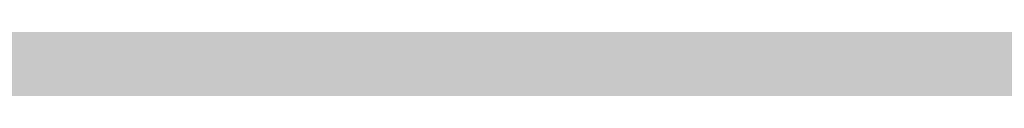
# Model space of a CAD drawing. Units: millimetres. Extents: x -22994 to 29398, y -19990 to 20176.
# Tile 95 of 135: x 229.428 to 230.597, y 84.498 to 84.556. Entities that reach past the tile are written whole.
import ezdxf
from ezdxf import colors
from ezdxf.entities.mleader import LeaderData, LeaderLine
from ezdxf.math import Vec2, Vec3

# ---------------------------------------------------------------- set-up
doc = ezdxf.new("R2010")
doc.units = ezdxf.units.MM
doc.header["$MEASUREMENT"] = 0
for name, color, linetype, lineweight in [('M-ANNO-TEXT', 7, 'Continuous', 25), ('M-DIMS', 2, 'Continuous', 18), ('M-EQPM-PATT', 7, 'Continuous', 18)]:
    doc.layers.add(name, color=color, linetype=linetype, lineweight=lineweight)
doc.styles.get("Standard").update_dxf_attribs({"font": 'arial.ttf'})
doc.dimstyles.get("Standard").update_dxf_attribs({"dimtxt": 0.18, "dimasz": 10000, "dimexe": 0.18, "dimexo": 0.0625, "dimgap": 0.09, "dimtad": 0, "dimtih": 1, "dimtoh": 1, "dimdec": 0, "dimzin": 0, "dimdsep": 46, "dimtxsty": 'Standard', "dimcen": 0.09, "dimadec": 0, "dimazin": 0, "dimtfac": 1, "dimtdec": 0, "dimtofl": 0, "dimtmove": 0, "dimatfit": 3, "dimfxl": 1, "dimtolj": 1, "dimtzin": 0, "dimlwd": 30, "dimarcsym": 0})

# ---------------------------------------------------------------- blocks, each defined once
blk = doc.blocks.new('*D2')
at = {"layer": 'Defpoints', "color": 0, "transparency": 16777216}
for p in [(6.6773, 10.2713), (290.852, 10.2713), (290.852, -5.0787)]:
    blk.add_point(p, dxfattribs=at)
at = {"layer": 'M-DIMS', "color": 0, "lineweight": -2, "transparency": 16777216}
for p, q in [((6.6773, 10.2088), (6.6773, -5.2587)), ((290.852, 10.2088), (290.852, -5.2587))]:
    blk.add_line(p, q, dxfattribs=at)
at = {"layer": 'M-DIMS', "color": 0, "lineweight": 30, "transparency": 16777216}
for p, q in [((-9993.3227, -5.0787), (-19993.3227, -5.0787)), ((10290.852, -5.0787), (20290.852, -5.0787))]:
    blk.add_line(p, q, dxfattribs=at)
at = {"layer": 'M-DIMS', "color": 0, "transparency": 16777216}
for points in [[(-9993.3227, 1661.5879), (-9993.3227, -1671.7454), (6.6773, -5.0787)], [(10290.852, 1661.5879), (10290.852, -1671.7454), (290.852, -5.0787)]]:
    blk.add_solid(points, dxfattribs=at)
at = {"layer": 'M-DIMS', "color": 0, "transparency": 16777216, "insert": (148.7647, -5.0787), "char_height": 0.18, "attachment_point": 5}
blk.add_mtext('\\A1;284.2', dxfattribs=at)
blk = doc.blocks.new('*D3')
at = {"layer": 'Defpoints', "color": 0, "transparency": 16777216}
for p in [(110.2647, 204.1654), (110.2647, 176.3662), (95.8327, 127.967)]:
    blk.add_point(p, dxfattribs=at)
at = {"layer": 'M-DIMS', "color": 0, "lineweight": -2, "transparency": 16777216}
for p, q in [((95.8327, 128.0295), (95.8327, 204.3454)), ((110.2647, 176.4287), (110.2647, 204.3454))]:
    blk.add_line(p, q, dxfattribs=at)
at = {"layer": 'M-DIMS', "color": 0, "lineweight": 30, "transparency": 16777216}
for p, q in [((-9904.1673, 204.1654), (-19904.1673, 204.1654)), ((10110.2647, 204.1654), (20110.2647, 204.1654))]:
    blk.add_line(p, q, dxfattribs=at)
at = {"layer": 'M-DIMS', "color": 0, "transparency": 16777216}
for points in [[(-9904.1673, 1870.8321), (-9904.1673, -1462.5013), (95.8327, 204.1654)], [(10110.2647, 1870.8321), (10110.2647, -1462.5013), (110.2647, 204.1654)]]:
    blk.add_solid(points, dxfattribs=at)
at = {"layer": 'M-DIMS', "color": 0, "transparency": 16777216, "insert": (103.0487, 204.1654), "char_height": 0.18, "attachment_point": 5}
blk.add_mtext('\\A1;14.432', dxfattribs=at)
blk = doc.blocks.new('*D4')
at = {"layer": 'Defpoints', "color": 0, "transparency": 16777216}
for p in [(116.2647, 204.1654), (110.2647, 176.3662), (116.2647, 176.3662)]:
    blk.add_point(p, dxfattribs=at)
at = {"layer": 'M-DIMS', "color": 0, "lineweight": -2, "transparency": 16777216}
for p, q in [((110.2647, 176.4287), (110.2647, 204.3454)), ((116.2647, 176.4287), (116.2647, 204.3454))]:
    blk.add_line(p, q, dxfattribs=at)
at = {"layer": 'M-DIMS', "color": 0, "lineweight": 30, "transparency": 16777216}
for p, q in [((-9889.7353, 204.1654), (-19889.7353, 204.1654)), ((10116.2647, 204.1654), (20116.2647, 204.1654))]:
    blk.add_line(p, q, dxfattribs=at)
at = {"layer": 'M-DIMS', "color": 0, "transparency": 16777216}
for points in [[(-9889.7353, 1870.8321), (-9889.7353, -1462.5013), (110.2647, 204.1654)], [(10116.2647, 1870.8321), (10116.2647, -1462.5013), (116.2647, 204.1654)]]:
    blk.add_solid(points, dxfattribs=at)
at = {"layer": 'M-DIMS', "color": 0, "transparency": 16777216, "insert": (113.2647, 204.1654), "char_height": 0.18, "attachment_point": 5}
blk.add_mtext('\\A1;6', dxfattribs=at)
blk = doc.blocks.new('*D5')
at = {"layer": 'Defpoints', "color": 0, "transparency": 16777216}
for p in [(181.2647, 204.1654), (116.2647, 176.3662), (181.2647, 176.3662)]:
    blk.add_point(p, dxfattribs=at)
at = {"layer": 'M-DIMS', "color": 0, "lineweight": -2, "transparency": 16777216}
for p, q in [((116.2647, 176.4287), (116.2647, 204.3454)), ((181.2647, 176.4287), (181.2647, 204.3454))]:
    blk.add_line(p, q, dxfattribs=at)
at = {"layer": 'M-DIMS', "color": 0, "lineweight": 30, "transparency": 16777216}
for p, q in [((-9883.7353, 204.1654), (-19883.7353, 204.1654)), ((10181.2647, 204.1654), (20181.2647, 204.1654))]:
    blk.add_line(p, q, dxfattribs=at)
at = {"layer": 'M-DIMS', "color": 0, "transparency": 16777216}
for points in [[(-9883.7353, 1870.8321), (-9883.7353, -1462.5013), (116.2647, 204.1654)], [(10181.2647, 1870.8321), (10181.2647, -1462.5013), (181.2647, 204.1654)]]:
    blk.add_solid(points, dxfattribs=at)
at = {"layer": 'M-DIMS', "color": 0, "transparency": 16777216, "insert": (148.7647, 204.1654), "char_height": 0.18, "attachment_point": 5}
blk.add_mtext('\\A1;65', dxfattribs=at)
blk = doc.blocks.new('*D6')
at = {"layer": 'Defpoints', "color": 0, "transparency": 16777216}
for p in [(187.2647, 204.1654), (181.2647, 176.3662), (187.2647, 176.3662)]:
    blk.add_point(p, dxfattribs=at)
at = {"layer": 'M-DIMS', "color": 0, "lineweight": -2, "transparency": 16777216}
for p, q in [((181.2647, 176.4287), (181.2647, 204.3454)), ((187.2647, 176.4287), (187.2647, 204.3454))]:
    blk.add_line(p, q, dxfattribs=at)
at = {"layer": 'M-DIMS', "color": 0, "lineweight": 30, "transparency": 16777216}
for p, q in [((-9818.7353, 204.1654), (-19818.7353, 204.1654)), ((10187.2647, 204.1654), (20187.2647, 204.1654))]:
    blk.add_line(p, q, dxfattribs=at)
at = {"layer": 'M-DIMS', "color": 0, "transparency": 16777216}
for points in [[(-9818.7353, 1870.8321), (-9818.7353, -1462.5013), (181.2647, 204.1654)], [(10187.2647, 1870.8321), (10187.2647, -1462.5013), (187.2647, 204.1654)]]:
    blk.add_solid(points, dxfattribs=at)
at = {"layer": 'M-DIMS', "color": 0, "transparency": 16777216, "insert": (184.2647, 204.1654), "char_height": 0.18, "attachment_point": 5}
blk.add_mtext('\\A1;6', dxfattribs=at)
blk = doc.blocks.new('*D7')
at = {"layer": 'Defpoints', "color": 0, "transparency": 16777216}
for p in [(201.6967, 204.1654), (187.2647, 176.3662), (201.6967, 127.967)]:
    blk.add_point(p, dxfattribs=at)
at = {"layer": 'M-DIMS', "color": 0, "lineweight": -2, "transparency": 16777216}
for p, q in [((187.2647, 176.4287), (187.2647, 204.3454)), ((201.6967, 128.0295), (201.6967, 204.3454))]:
    blk.add_line(p, q, dxfattribs=at)
at = {"layer": 'M-DIMS', "color": 0, "lineweight": 30, "transparency": 16777216}
for p, q in [((-9812.7353, 204.1654), (-19812.7353, 204.1654)), ((10201.6967, 204.1654), (20201.6967, 204.1654))]:
    blk.add_line(p, q, dxfattribs=at)
at = {"layer": 'M-DIMS', "color": 0, "transparency": 16777216}
for points in [[(-9812.7353, 1870.8321), (-9812.7353, -1462.5013), (187.2647, 204.1654)], [(10201.6967, 1870.8321), (10201.6967, -1462.5013), (201.6967, 204.1654)]]:
    blk.add_solid(points, dxfattribs=at)
at = {"layer": 'M-DIMS', "color": 0, "transparency": 16777216, "insert": (194.4807, 204.1654), "char_height": 0.18, "attachment_point": 5}
blk.add_mtext('\\A1;14.432', dxfattribs=at)
blk = doc.blocks.new('*D8')
at = {"layer": 'Defpoints', "color": 0, "transparency": 16777216}
for p in [(227.6485, 204.1654), (227.6485, 146.7296), (201.6967, 127.967)]:
    blk.add_point(p, dxfattribs=at)
at = {"layer": 'M-DIMS', "color": 0, "lineweight": -2, "transparency": 16777216}
for p, q in [((201.6967, 128.0295), (201.6967, 204.3454)), ((227.6485, 146.7921), (227.6485, 204.3454))]:
    blk.add_line(p, q, dxfattribs=at)
at = {"layer": 'M-DIMS', "color": 0, "lineweight": 30, "transparency": 16777216}
for p, q in [((-9798.3033, 204.1654), (-19798.3033, 204.1654)), ((10227.6485, 204.1654), (20227.6485, 204.1654))]:
    blk.add_line(p, q, dxfattribs=at)
at = {"layer": 'M-DIMS', "color": 0, "transparency": 16777216}
for points in [[(-9798.3033, 1870.8321), (-9798.3033, -1462.5013), (201.6967, 204.1654)], [(10227.6485, 1870.8321), (10227.6485, -1462.5013), (227.6485, 204.1654)]]:
    blk.add_solid(points, dxfattribs=at)
at = {"layer": 'M-DIMS', "color": 0, "transparency": 16777216, "insert": (214.6726, 204.1654), "char_height": 0.18, "attachment_point": 5}
blk.add_mtext('\\A1;25.95', dxfattribs=at)
blk = doc.blocks.new('*D9')
at = {"layer": 'Defpoints', "color": 0, "transparency": 16777216}
for p in [(187.2647, 176.3662), (306.202, 176.3662), (290.852, 10.2713)]:
    blk.add_point(p, dxfattribs=at)
at = {"layer": 'M-DIMS', "color": 0, "lineweight": 30, "transparency": 16777216}
for p, q in [((306.202, 10176.3662), (306.202, 20176.3662)), ((306.202, -9989.7287), (306.202, -19989.7287))]:
    blk.add_line(p, q, dxfattribs=at)
at = {"layer": 'M-DIMS', "color": 0, "lineweight": -2, "transparency": 16777216}
for p, q in [((187.3272, 176.3662), (306.382, 176.3662)), ((290.9145, 10.2713), (306.382, 10.2713))]:
    blk.add_line(p, q, dxfattribs=at)
at = {"layer": 'M-DIMS', "color": 0, "transparency": 16777216}
for points in [[(-1360.4646, 10176.3662), (1972.8687, 10176.3662), (306.202, 176.3662)], [(-1360.4646, -9989.7287), (1972.8687, -9989.7287), (306.202, 10.2713)]]:
    blk.add_solid(points, dxfattribs=at)
at = {"layer": 'M-DIMS', "color": 0, "transparency": 16777216, "insert": (306.202, 93.3187), "char_height": 0.18, "attachment_point": 5}
blk.add_mtext('\\A1;166.1', dxfattribs=at)
blk = doc.blocks.new('*D10')
at = {"layer": 'Defpoints', "color": 0, "transparency": 16777216}
for p in [(125.6498, 136.0713), (133.3459, 136.0713), (133.3459, -5.0787)]:
    blk.add_point(p, dxfattribs=at)
at = {"layer": 'M-DIMS', "color": 0, "lineweight": -2, "transparency": 16777216}
for p, q in [((125.6498, 136.0088), (125.6498, -5.2587)), ((133.3459, 136.0088), (133.3459, -5.2587))]:
    blk.add_line(p, q, dxfattribs=at)
at = {"layer": 'M-DIMS', "color": 0, "lineweight": 30, "transparency": 16777216}
for p, q in [((-9874.3502, -5.0787), (-19874.3502, -5.0787)), ((10133.3459, -5.0787), (20133.3459, -5.0787))]:
    blk.add_line(p, q, dxfattribs=at)
at = {"layer": 'M-DIMS', "color": 0, "transparency": 16777216}
for points in [[(-9874.3502, 1661.5879), (-9874.3502, -1671.7454), (125.6498, -5.0787)], [(10133.3459, 1661.5879), (10133.3459, -1671.7454), (133.3459, -5.0787)]]:
    blk.add_solid(points, dxfattribs=at)
at = {"layer": 'M-DIMS', "color": 0, "transparency": 16777216, "insert": (129.4978, -5.0787), "char_height": 0.18, "attachment_point": 5}
blk.add_mtext('\\A1;7.696', dxfattribs=at)
blk = doc.blocks.new('*D11')
at = {"layer": 'Defpoints', "color": 0, "transparency": 16777216}
for p in [(133.3459, 136.0713), (135.6498, 136.0713), (135.6498, -5.0787)]:
    blk.add_point(p, dxfattribs=at)
at = {"layer": 'M-DIMS', "color": 0, "lineweight": -2, "transparency": 16777216}
for p, q in [((133.3459, 136.0088), (133.3459, -5.2587)), ((135.6498, 136.0088), (135.6498, -5.2587))]:
    blk.add_line(p, q, dxfattribs=at)
at = {"layer": 'M-DIMS', "color": 0, "lineweight": 30, "transparency": 16777216}
for p, q in [((-9866.6541, -5.0787), (-19866.6541, -5.0787)), ((10135.6498, -5.0787), (20135.6498, -5.0787))]:
    blk.add_line(p, q, dxfattribs=at)
at = {"layer": 'M-DIMS', "color": 0, "transparency": 16777216}
for points in [[(-9866.6541, 1661.5879), (-9866.6541, -1671.7454), (133.3459, -5.0787)], [(10135.6498, 1661.5879), (10135.6498, -1671.7454), (135.6498, -5.0787)]]:
    blk.add_solid(points, dxfattribs=at)
at = {"layer": 'M-DIMS', "color": 0, "transparency": 16777216, "insert": (134.4978, -5.0787), "char_height": 0.18, "attachment_point": 5}
blk.add_mtext('\\A1;2.304', dxfattribs=at)
blk = doc.blocks.new('*D12')
at = {"layer": 'Defpoints', "color": 0, "transparency": 16777216}
for p in [(135.6498, 136.0713), (145.6498, 136.0713), (145.6498, -5.0787)]:
    blk.add_point(p, dxfattribs=at)
at = {"layer": 'M-DIMS', "color": 0, "lineweight": -2, "transparency": 16777216}
for p, q in [((135.6498, 136.0088), (135.6498, -5.2587)), ((145.6498, 136.0088), (145.6498, -5.2587))]:
    blk.add_line(p, q, dxfattribs=at)
at = {"layer": 'M-DIMS', "color": 0, "lineweight": 30, "transparency": 16777216}
for p, q in [((-9864.3502, -5.0787), (-19864.3502, -5.0787)), ((10145.6498, -5.0787), (20145.6498, -5.0787))]:
    blk.add_line(p, q, dxfattribs=at)
at = {"layer": 'M-DIMS', "color": 0, "transparency": 16777216}
for points in [[(-9864.3502, 1661.5879), (-9864.3502, -1671.7454), (135.6498, -5.0787)], [(10145.6498, 1661.5879), (10145.6498, -1671.7454), (145.6498, -5.0787)]]:
    blk.add_solid(points, dxfattribs=at)
at = {"layer": 'M-DIMS', "color": 0, "transparency": 16777216, "insert": (140.6498, -5.0787), "char_height": 0.18, "attachment_point": 5}
blk.add_mtext('\\A1;10', dxfattribs=at)
blk = doc.blocks.new('*D13')
at = {"layer": 'Defpoints', "color": 0, "transparency": 16777216}
for p in [(145.6498, 136.0713), (155.6498, 136.0713), (155.6498, -5.0787)]:
    blk.add_point(p, dxfattribs=at)
at = {"layer": 'M-DIMS', "color": 0, "lineweight": -2, "transparency": 16777216}
for p, q in [((145.6498, 136.0088), (145.6498, -5.2587)), ((155.6498, 136.0088), (155.6498, -5.2587))]:
    blk.add_line(p, q, dxfattribs=at)
at = {"layer": 'M-DIMS', "color": 0, "lineweight": 30, "transparency": 16777216}
for p, q in [((-9854.3502, -5.0787), (-19854.3502, -5.0787)), ((10155.6498, -5.0787), (20155.6498, -5.0787))]:
    blk.add_line(p, q, dxfattribs=at)
at = {"layer": 'M-DIMS', "color": 0, "transparency": 16777216}
for points in [[(-9854.3502, 1661.5879), (-9854.3502, -1671.7454), (145.6498, -5.0787)], [(10155.6498, 1661.5879), (10155.6498, -1671.7454), (155.6498, -5.0787)]]:
    blk.add_solid(points, dxfattribs=at)
at = {"layer": 'M-DIMS', "color": 0, "transparency": 16777216, "insert": (150.6498, -5.0787), "char_height": 0.18, "attachment_point": 5}
blk.add_mtext('\\A1;10', dxfattribs=at)
blk = doc.blocks.new('*D14')
at = {"layer": 'Defpoints', "color": 0, "transparency": 16777216}
for p in [(155.6498, 136.0713), (165.6498, 136.0713), (165.6498, -5.0787)]:
    blk.add_point(p, dxfattribs=at)
at = {"layer": 'M-DIMS', "color": 0, "lineweight": -2, "transparency": 16777216}
for p, q in [((155.6498, 136.0088), (155.6498, -5.2587)), ((165.6498, 136.0088), (165.6498, -5.2587))]:
    blk.add_line(p, q, dxfattribs=at)
at = {"layer": 'M-DIMS', "color": 0, "lineweight": 30, "transparency": 16777216}
for p, q in [((-9844.3502, -5.0787), (-19844.3502, -5.0787)), ((10165.6498, -5.0787), (20165.6498, -5.0787))]:
    blk.add_line(p, q, dxfattribs=at)
at = {"layer": 'M-DIMS', "color": 0, "transparency": 16777216}
for points in [[(-9844.3502, 1661.5879), (-9844.3502, -1671.7454), (155.6498, -5.0787)], [(10165.6498, 1661.5879), (10165.6498, -1671.7454), (165.6498, -5.0787)]]:
    blk.add_solid(points, dxfattribs=at)
at = {"layer": 'M-DIMS', "color": 0, "transparency": 16777216, "insert": (160.6498, -5.0787), "char_height": 0.18, "attachment_point": 5}
blk.add_mtext('\\A1;10', dxfattribs=at)
blk = doc.blocks.new('*D15')
at = {"layer": 'Defpoints', "color": 0, "transparency": 16777216}
for p in [(173.3459, 154.788), (173.3459, 136.0713), (306.202, 136.0713)]:
    blk.add_point(p, dxfattribs=at)
at = {"layer": 'M-DIMS', "color": 0, "lineweight": 30, "transparency": 16777216}
for p, q in [((306.202, 10154.788), (306.202, 20154.788)), ((306.202, -9863.9287), (306.202, -19863.9287))]:
    blk.add_line(p, q, dxfattribs=at)
at = {"layer": 'M-DIMS', "color": 0, "lineweight": -2, "transparency": 16777216}
for p, q in [((173.4084, 154.788), (306.382, 154.788)), ((173.4084, 136.0713), (306.382, 136.0713))]:
    blk.add_line(p, q, dxfattribs=at)
at = {"layer": 'M-DIMS', "color": 0, "transparency": 16777216}
for points in [[(-1360.4646, 10154.788), (1972.8687, 10154.788), (306.202, 154.788)], [(-1360.4646, -9863.9287), (1972.8687, -9863.9287), (306.202, 136.0713)]]:
    blk.add_solid(points, dxfattribs=at)
at = {"layer": 'M-DIMS', "color": 0, "transparency": 16777216, "insert": (306.202, 145.4297), "char_height": 0.18, "attachment_point": 5}
blk.add_mtext('\\A1;18.717', dxfattribs=at)
blk = doc.blocks.new('*D16')
at = {"layer": 'Defpoints', "color": 0, "transparency": 16777216}
for p in [(120.1702, 204.1654), (110.4658, 48.0349), (120.1702, 48.0349)]:
    blk.add_point(p, dxfattribs=at)
at = {"layer": 'M-DIMS', "color": 0, "lineweight": -2, "transparency": 16777216}
for p, q in [((110.4658, 48.0974), (110.4658, 204.3454)), ((120.1702, 48.0974), (120.1702, 204.3454))]:
    blk.add_line(p, q, dxfattribs=at)
at = {"layer": 'M-DIMS', "color": 0, "lineweight": 30, "transparency": 16777216}
for p, q in [((-9889.5342, 204.1654), (-19889.5342, 204.1654)), ((10120.1702, 204.1654), (20120.1702, 204.1654))]:
    blk.add_line(p, q, dxfattribs=at)
at = {"layer": 'M-DIMS', "color": 0, "transparency": 16777216}
for points in [[(-9889.5342, 1870.8321), (-9889.5342, -1462.5013), (110.4658, 204.1654)], [(10120.1702, 1870.8321), (10120.1702, -1462.5013), (120.1702, 204.1654)]]:
    blk.add_solid(points, dxfattribs=at)
at = {"layer": 'M-DIMS', "color": 0, "transparency": 16777216, "insert": (115.318, 204.1654), "char_height": 0.18, "attachment_point": 5}
blk.add_mtext('\\A1;9.704', dxfattribs=at)
blk = doc.blocks.new('*D17')
at = {"layer": 'Defpoints', "color": 0, "transparency": 16777216}
for p in [(126.1702, 204.1654), (120.1702, 48.0349), (126.1702, 48.0349)]:
    blk.add_point(p, dxfattribs=at)
at = {"layer": 'M-DIMS', "color": 0, "lineweight": -2, "transparency": 16777216}
for p, q in [((120.1702, 48.0974), (120.1702, 204.3454)), ((126.1702, 48.0974), (126.1702, 204.3454))]:
    blk.add_line(p, q, dxfattribs=at)
at = {"layer": 'M-DIMS', "color": 0, "lineweight": 30, "transparency": 16777216}
for p, q in [((-9879.8298, 204.1654), (-19879.8298, 204.1654)), ((10126.1702, 204.1654), (20126.1702, 204.1654))]:
    blk.add_line(p, q, dxfattribs=at)
at = {"layer": 'M-DIMS', "color": 0, "transparency": 16777216}
for points in [[(-9879.8298, 1870.8321), (-9879.8298, -1462.5013), (120.1702, 204.1654)], [(10126.1702, 1870.8321), (10126.1702, -1462.5013), (126.1702, 204.1654)]]:
    blk.add_solid(points, dxfattribs=at)
at = {"layer": 'M-DIMS', "color": 0, "transparency": 16777216, "insert": (123.1702, 204.1654), "char_height": 0.18, "attachment_point": 5}
blk.add_mtext('\\A1;6', dxfattribs=at)
blk = doc.blocks.new('*D18')
at = {"layer": 'Defpoints', "color": 0, "transparency": 16777216}
for p in [(132.1702, 204.1654), (126.1702, 48.0349), (132.1702, 48.0349)]:
    blk.add_point(p, dxfattribs=at)
at = {"layer": 'M-DIMS', "color": 0, "lineweight": -2, "transparency": 16777216}
for p, q in [((126.1702, 48.0974), (126.1702, 204.3454)), ((132.1702, 48.0974), (132.1702, 204.3454))]:
    blk.add_line(p, q, dxfattribs=at)
at = {"layer": 'M-DIMS', "color": 0, "lineweight": 30, "transparency": 16777216}
for p, q in [((-9873.8298, 204.1654), (-19873.8298, 204.1654)), ((10132.1702, 204.1654), (20132.1702, 204.1654))]:
    blk.add_line(p, q, dxfattribs=at)
at = {"layer": 'M-DIMS', "color": 0, "transparency": 16777216}
for points in [[(-9873.8298, 1870.8321), (-9873.8298, -1462.5013), (126.1702, 204.1654)], [(10132.1702, 1870.8321), (10132.1702, -1462.5013), (132.1702, 204.1654)]]:
    blk.add_solid(points, dxfattribs=at)
at = {"layer": 'M-DIMS', "color": 0, "transparency": 16777216, "insert": (129.1702, 204.1654), "char_height": 0.18, "attachment_point": 5}
blk.add_mtext('\\A1;6', dxfattribs=at)
blk = doc.blocks.new('*D19')
at = {"layer": 'Defpoints', "color": 0, "transparency": 16777216}
for p in [(138.1702, 204.1654), (132.1702, 48.0349), (138.1702, 48.0349)]:
    blk.add_point(p, dxfattribs=at)
at = {"layer": 'M-DIMS', "color": 0, "lineweight": -2, "transparency": 16777216}
for p, q in [((132.1702, 48.0974), (132.1702, 204.3454)), ((138.1702, 48.0974), (138.1702, 204.3454))]:
    blk.add_line(p, q, dxfattribs=at)
at = {"layer": 'M-DIMS', "color": 0, "lineweight": 30, "transparency": 16777216}
for p, q in [((-9867.8298, 204.1654), (-19867.8298, 204.1654)), ((10138.1702, 204.1654), (20138.1702, 204.1654))]:
    blk.add_line(p, q, dxfattribs=at)
at = {"layer": 'M-DIMS', "color": 0, "transparency": 16777216}
for points in [[(-9867.8298, 1870.8321), (-9867.8298, -1462.5013), (132.1702, 204.1654)], [(10138.1702, 1870.8321), (10138.1702, -1462.5013), (138.1702, 204.1654)]]:
    blk.add_solid(points, dxfattribs=at)
at = {"layer": 'M-DIMS', "color": 0, "transparency": 16777216, "insert": (135.1702, 204.1654), "char_height": 0.18, "attachment_point": 5}
blk.add_mtext('\\A1;6', dxfattribs=at)
blk = doc.blocks.new('*D20')
at = {"layer": 'Defpoints', "color": 0, "transparency": 16777216}
for p in [(144.1702, 204.1654), (138.1702, 48.0349), (144.1702, 48.0349)]:
    blk.add_point(p, dxfattribs=at)
at = {"layer": 'M-DIMS', "color": 0, "lineweight": -2, "transparency": 16777216}
for p, q in [((138.1702, 48.0974), (138.1702, 204.3454)), ((144.1702, 48.0974), (144.1702, 204.3454))]:
    blk.add_line(p, q, dxfattribs=at)
at = {"layer": 'M-DIMS', "color": 0, "lineweight": 30, "transparency": 16777216}
for p, q in [((-9861.8298, 204.1654), (-19861.8298, 204.1654)), ((10144.1702, 204.1654), (20144.1702, 204.1654))]:
    blk.add_line(p, q, dxfattribs=at)
at = {"layer": 'M-DIMS', "color": 0, "transparency": 16777216}
for points in [[(-9861.8298, 1870.8321), (-9861.8298, -1462.5013), (138.1702, 204.1654)], [(10144.1702, 1870.8321), (10144.1702, -1462.5013), (144.1702, 204.1654)]]:
    blk.add_solid(points, dxfattribs=at)
at = {"layer": 'M-DIMS', "color": 0, "transparency": 16777216, "insert": (141.1702, 204.1654), "char_height": 0.18, "attachment_point": 5}
blk.add_mtext('\\A1;6', dxfattribs=at)
blk = doc.blocks.new('*D21')
at = {"layer": 'Defpoints', "color": 0, "transparency": 16777216}
for p in [(149.1157, 204.1654), (144.1702, 48.0349), (149.1157, 48.0349)]:
    blk.add_point(p, dxfattribs=at)
at = {"layer": 'M-DIMS', "color": 0, "lineweight": -2, "transparency": 16777216}
for p, q in [((144.1702, 48.0974), (144.1702, 204.3454)), ((149.1157, 48.0974), (149.1157, 204.3454))]:
    blk.add_line(p, q, dxfattribs=at)
at = {"layer": 'M-DIMS', "color": 0, "lineweight": 30, "transparency": 16777216}
for p, q in [((-9855.8298, 204.1654), (-19855.8298, 204.1654)), ((10149.1157, 204.1654), (20149.1157, 204.1654))]:
    blk.add_line(p, q, dxfattribs=at)
at = {"layer": 'M-DIMS', "color": 0, "transparency": 16777216}
for points in [[(-9855.8298, 1870.8321), (-9855.8298, -1462.5013), (144.1702, 204.1654)], [(10149.1157, 1870.8321), (10149.1157, -1462.5013), (149.1157, 204.1654)]]:
    blk.add_solid(points, dxfattribs=at)
at = {"layer": 'M-DIMS', "color": 0, "transparency": 16777216, "insert": (146.6429, 204.1654), "char_height": 0.18, "attachment_point": 5}
blk.add_mtext('\\A1;4.945', dxfattribs=at)
blk = doc.blocks.new('*D22')
at = {"layer": 'Defpoints', "color": 0, "transparency": 16777216}
for p in [(149.1157, 30.9895), (155.1157, 30.9895), (155.1157, -5.0787)]:
    blk.add_point(p, dxfattribs=at)
at = {"layer": 'M-DIMS', "color": 0, "lineweight": -2, "transparency": 16777216}
for p, q in [((149.1157, 30.927), (149.1157, -5.2587)), ((155.1157, 30.927), (155.1157, -5.2587))]:
    blk.add_line(p, q, dxfattribs=at)
at = {"layer": 'M-DIMS', "color": 0, "lineweight": 30, "transparency": 16777216}
for p, q in [((-9850.8843, -5.0787), (-19850.8843, -5.0787)), ((10155.1157, -5.0787), (20155.1157, -5.0787))]:
    blk.add_line(p, q, dxfattribs=at)
at = {"layer": 'M-DIMS', "color": 0, "transparency": 16777216}
for points in [[(-9850.8843, 1661.5879), (-9850.8843, -1671.7454), (149.1157, -5.0787)], [(10155.1157, 1661.5879), (10155.1157, -1671.7454), (155.1157, -5.0787)]]:
    blk.add_solid(points, dxfattribs=at)
at = {"layer": 'M-DIMS', "color": 0, "transparency": 16777216, "insert": (152.1157, -5.0787), "char_height": 0.18, "attachment_point": 5}
blk.add_mtext('\\A1;6', dxfattribs=at)
blk = doc.blocks.new('*D23')
at = {"layer": 'Defpoints', "color": 0, "transparency": 16777216}
for p in [(155.1157, 30.9895), (161.1157, 30.9895), (161.1157, -5.0787)]:
    blk.add_point(p, dxfattribs=at)
at = {"layer": 'M-DIMS', "color": 0, "lineweight": -2, "transparency": 16777216}
for p, q in [((155.1157, 30.927), (155.1157, -5.2587)), ((161.1157, 30.927), (161.1157, -5.2587))]:
    blk.add_line(p, q, dxfattribs=at)
at = {"layer": 'M-DIMS', "color": 0, "lineweight": 30, "transparency": 16777216}
for p, q in [((-9844.8843, -5.0787), (-19844.8843, -5.0787)), ((10161.1157, -5.0787), (20161.1157, -5.0787))]:
    blk.add_line(p, q, dxfattribs=at)
at = {"layer": 'M-DIMS', "color": 0, "transparency": 16777216}
for points in [[(-9844.8843, 1661.5879), (-9844.8843, -1671.7454), (155.1157, -5.0787)], [(10161.1157, 1661.5879), (10161.1157, -1671.7454), (161.1157, -5.0787)]]:
    blk.add_solid(points, dxfattribs=at)
at = {"layer": 'M-DIMS', "color": 0, "transparency": 16777216, "insert": (158.1157, -5.0787), "char_height": 0.18, "attachment_point": 5}
blk.add_mtext('\\A1;6', dxfattribs=at)
blk = doc.blocks.new('*D24')
at = {"layer": 'Defpoints', "color": 0, "transparency": 16777216}
for p in [(161.1157, 30.9895), (166.4387, 30.9895), (166.4387, -5.0787)]:
    blk.add_point(p, dxfattribs=at)
at = {"layer": 'M-DIMS', "color": 0, "lineweight": -2, "transparency": 16777216}
for p, q in [((161.1157, 30.927), (161.1157, -5.2587)), ((166.4387, 30.927), (166.4387, -5.2587))]:
    blk.add_line(p, q, dxfattribs=at)
at = {"layer": 'M-DIMS', "color": 0, "lineweight": 30, "transparency": 16777216}
for p, q in [((-9838.8843, -5.0787), (-19838.8843, -5.0787)), ((10166.4387, -5.0787), (20166.4387, -5.0787))]:
    blk.add_line(p, q, dxfattribs=at)
at = {"layer": 'M-DIMS', "color": 0, "transparency": 16777216}
for points in [[(-9838.8843, 1661.5879), (-9838.8843, -1671.7454), (161.1157, -5.0787)], [(10166.4387, 1661.5879), (10166.4387, -1671.7454), (166.4387, -5.0787)]]:
    blk.add_solid(points, dxfattribs=at)
at = {"layer": 'M-DIMS', "color": 0, "transparency": 16777216, "insert": (163.7772, -5.0787), "char_height": 0.18, "attachment_point": 5}
blk.add_mtext('\\A1;5.323', dxfattribs=at)
blk = doc.blocks.new('*D25')
at = {"layer": 'Defpoints', "color": 0, "transparency": 16777216}
for p in [(166.4387, 30.9895), (172.4387, 30.9895), (172.4387, -5.0787)]:
    blk.add_point(p, dxfattribs=at)
at = {"layer": 'M-DIMS', "color": 0, "lineweight": -2, "transparency": 16777216}
for p, q in [((166.4387, 30.927), (166.4387, -5.2587)), ((172.4387, 30.927), (172.4387, -5.2587))]:
    blk.add_line(p, q, dxfattribs=at)
at = {"layer": 'M-DIMS', "color": 0, "lineweight": 30, "transparency": 16777216}
for p, q in [((-9833.5613, -5.0787), (-19833.5613, -5.0787)), ((10172.4387, -5.0787), (20172.4387, -5.0787))]:
    blk.add_line(p, q, dxfattribs=at)
at = {"layer": 'M-DIMS', "color": 0, "transparency": 16777216}
for points in [[(-9833.5613, 1661.5879), (-9833.5613, -1671.7454), (166.4387, -5.0787)], [(10172.4387, 1661.5879), (10172.4387, -1671.7454), (172.4387, -5.0787)]]:
    blk.add_solid(points, dxfattribs=at)
at = {"layer": 'M-DIMS', "color": 0, "transparency": 16777216, "insert": (169.4387, -5.0787), "char_height": 0.18, "attachment_point": 5}
blk.add_mtext('\\A1;6', dxfattribs=at)
blk = doc.blocks.new('*D26')
at = {"layer": 'Defpoints', "color": 0, "transparency": 16777216}
for p in [(172.4387, 30.9895), (178.4387, 30.9895), (178.4387, -5.0787)]:
    blk.add_point(p, dxfattribs=at)
at = {"layer": 'M-DIMS', "color": 0, "lineweight": -2, "transparency": 16777216}
for p, q in [((172.4387, 30.927), (172.4387, -5.2587)), ((178.4387, 30.927), (178.4387, -5.2587))]:
    blk.add_line(p, q, dxfattribs=at)
at = {"layer": 'M-DIMS', "color": 0, "lineweight": 30, "transparency": 16777216}
for p, q in [((-9827.5613, -5.0787), (-19827.5613, -5.0787)), ((10178.4387, -5.0787), (20178.4387, -5.0787))]:
    blk.add_line(p, q, dxfattribs=at)
at = {"layer": 'M-DIMS', "color": 0, "transparency": 16777216}
for points in [[(-9827.5613, 1661.5879), (-9827.5613, -1671.7454), (172.4387, -5.0787)], [(10178.4387, 1661.5879), (10178.4387, -1671.7454), (178.4387, -5.0787)]]:
    blk.add_solid(points, dxfattribs=at)
at = {"layer": 'M-DIMS', "color": 0, "transparency": 16777216, "insert": (175.4387, -5.0787), "char_height": 0.18, "attachment_point": 5}
blk.add_mtext('\\A1;6', dxfattribs=at)
blk = doc.blocks.new('*D27')
at = {"layer": 'Defpoints', "color": 0, "transparency": 16777216}
for p in [(178.4387, 30.9895), (188.1175, 30.9895), (188.1175, -5.0787)]:
    blk.add_point(p, dxfattribs=at)
at = {"layer": 'M-DIMS', "color": 0, "lineweight": -2, "transparency": 16777216}
for p, q in [((178.4387, 30.927), (178.4387, -5.2587)), ((188.1175, 30.927), (188.1175, -5.2587))]:
    blk.add_line(p, q, dxfattribs=at)
at = {"layer": 'M-DIMS', "color": 0, "lineweight": 30, "transparency": 16777216}
for p, q in [((-9821.5613, -5.0787), (-19821.5613, -5.0787)), ((10188.1175, -5.0787), (20188.1175, -5.0787))]:
    blk.add_line(p, q, dxfattribs=at)
at = {"layer": 'M-DIMS', "color": 0, "transparency": 16777216}
for points in [[(-9821.5613, 1661.5879), (-9821.5613, -1671.7454), (178.4387, -5.0787)], [(10188.1175, 1661.5879), (10188.1175, -1671.7454), (188.1175, -5.0787)]]:
    blk.add_solid(points, dxfattribs=at)
at = {"layer": 'M-DIMS', "color": 0, "transparency": 16777216, "insert": (183.2781, -5.0787), "char_height": 0.18, "attachment_point": 5}
blk.add_mtext('\\A1;9.679', dxfattribs=at)
blk = doc.blocks.new('*D28')
at = {"layer": 'Defpoints', "color": 0, "transparency": 16777216}
for p in [(188.1175, 48.0349), (306.202, 48.0349), (188.1175, 30.9895)]:
    blk.add_point(p, dxfattribs=at)
at = {"layer": 'M-DIMS', "color": 0, "lineweight": 30, "transparency": 16777216}
for p, q in [((306.202, 10048.0349), (306.202, 20048.0349)), ((306.202, -9969.0105), (306.202, -19969.0105))]:
    blk.add_line(p, q, dxfattribs=at)
at = {"layer": 'M-DIMS', "color": 0, "lineweight": -2, "transparency": 16777216}
for p, q in [((188.18, 48.0349), (306.382, 48.0349)), ((188.18, 30.9895), (306.382, 30.9895))]:
    blk.add_line(p, q, dxfattribs=at)
at = {"layer": 'M-DIMS', "color": 0, "transparency": 16777216}
for points in [[(-1360.4646, 10048.0349), (1972.8687, 10048.0349), (306.202, 48.0349)], [(-1360.4646, -9969.0105), (1972.8687, -9969.0105), (306.202, 30.9895)]]:
    blk.add_solid(points, dxfattribs=at)
at = {"layer": 'M-DIMS', "color": 0, "transparency": 16777216, "insert": (306.202, 39.5122), "char_height": 0.18, "attachment_point": 5}
blk.add_mtext('\\A1;17.045', dxfattribs=at)
blk = doc.blocks.new('*D29')
at = {"layer": 'Defpoints', "color": 0, "transparency": 16777216}
for p in [(36.8006, 80.045), (64.0296, 80.045)]:
    blk.add_point(p, dxfattribs=at)
at = {"layer": 'M-DIMS', "color": 0, "lineweight": -2, "transparency": 16777216}
for p, q in [((50.4151, 79.955), (50.4151, 80.135)), ((50.3251, 80.045), (50.5051, 80.045))]:
    blk.add_line(p, q, dxfattribs=at)
at = {"layer": 'M-DIMS', "color": 0, "lineweight": 30, "transparency": 16777216}
blk.add_line((20064.0296, 80.0303), (10064.0296, 80.0377), dxfattribs=at)
at = {"layer": 'M-DIMS', "color": 0, "transparency": 16777216}
blk.add_solid([(10064.0309, 1746.7043), (10064.0284, -1586.629), (64.0296, 80.045)], dxfattribs=at)
at = {"layer": 'M-DIMS', "color": 0, "transparency": 16777216, "insert": (20064.5213, 80.0303), "char_height": 0.18, "attachment_point": 5}
blk.add_mtext('\\A1;∅27.23', dxfattribs=at)
blk = doc.blocks.new('*D30')
at = {"layer": 'Defpoints', "color": 0, "transparency": 16777216}
for p in [(216.3148, 146.7291), (238.9821, 146.73)]:
    blk.add_point(p, dxfattribs=at)
at = {"layer": 'M-DIMS', "color": 0, "lineweight": 30, "transparency": 16777216}
blk.add_line((20238.9821, 147.4959), (10238.9821, 147.1129), dxfattribs=at)
at = {"layer": 'M-DIMS', "color": 0, "lineweight": -2, "transparency": 16777216}
for p, q in [((227.6485, 146.6396), (227.6485, 146.8196)), ((227.5585, 146.7296), (227.7385, 146.7296))]:
    blk.add_line(p, q, dxfattribs=at)
at = {"layer": 'M-DIMS', "color": 0, "transparency": 16777216}
blk.add_solid([(10238.9183, 1813.7796), (10239.0459, -1519.5537), (238.9821, 146.73)], dxfattribs=at)
at = {"layer": 'M-DIMS', "color": 0, "transparency": 16777216, "insert": (20239.5436, 147.4959), "char_height": 0.18, "attachment_point": 5}
blk.add_mtext('\\A1;∅22.667', dxfattribs=at)
blk = doc.blocks.new('*D31')
at = {"layer": 'Defpoints', "color": 0, "transparency": 16777216}
for p in [(223.1641, 146.7291), (232.1328, 146.73)]:
    blk.add_point(p, dxfattribs=at)
at = {"layer": 'M-DIMS', "color": 0, "lineweight": 30, "transparency": 16777216}
blk.add_line((20232.1327, 148.6656), (10232.1328, 147.6978), dxfattribs=at)
at = {"layer": 'M-DIMS', "color": 0, "lineweight": -2, "transparency": 16777216}
for p, q in [((227.6485, 146.6396), (227.6485, 146.8196)), ((227.5585, 146.7296), (227.7385, 146.7296))]:
    blk.add_line(p, q, dxfattribs=at)
at = {"layer": 'M-DIMS', "color": 0, "transparency": 16777216}
blk.add_solid([(10231.9715, 1814.3645), (10232.2941, -1518.9688), (232.1328, 146.73)], dxfattribs=at)
at = {"layer": 'M-DIMS', "color": 0, "transparency": 16777216, "insert": (20232.6245, 148.6656), "char_height": 0.18, "attachment_point": 5}
blk.add_mtext('\\A1;∅8.969', dxfattribs=at)
blk = doc.blocks.new('*D33')
at = {"layer": 'Defpoints', "color": 0, "transparency": 16777216}
for p in [(229.5613, 154.3773), (232.9972, 153.3509)]:
    blk.add_point(p, dxfattribs=at)
at = {"layer": 'M-DIMS', "color": 0, "lineweight": -2, "transparency": 16777216}
for p, q in [((229.5613, 154.2873), (229.5613, 154.4673)), ((229.4713, 154.3773), (229.6513, 154.3773))]:
    blk.add_line(p, q, dxfattribs=at)
at = {"layer": 'M-DIMS', "color": 0, "lineweight": 30, "transparency": 16777216}
for p, q in [((19396.3388, -5570.8378), (9814.668, -2708.7434)), ((29396.3388, -5570.8378), (19396.3388, -5570.8378))]:
    blk.add_line(p, q, dxfattribs=at)
at = {"layer": 'M-DIMS', "color": 0, "transparency": 16777216}
blk.add_solid([(10291.6837, -1111.7983), (9337.6523, -4305.6886), (232.9972, 153.3509)], dxfattribs=at)
at = {"layer": 'M-DIMS', "color": 0, "transparency": 16777216, "insert": (29397.0125, -5570.8378), "char_height": 0.18, "attachment_point": 5}
blk.add_mtext('\\A1;6X R3.586', dxfattribs=at)
blk = doc.blocks.new('*D36')
at = {"layer": 'Defpoints', "color": 0, "transparency": 16777216}
for p in [(46.39, 31.3035), (46.3875, 26.5934)]:
    blk.add_point(p, dxfattribs=at)
at = {"layer": 'M-DIMS', "color": 0, "lineweight": 30, "transparency": 16777216}
for p, q in [((57.1499, 20031.3006), (51.77, 10031.302)), ((10057.1499, 20031.3006), (57.1499, 20031.3006))]:
    blk.add_line(p, q, dxfattribs=at)
at = {"layer": 'M-DIMS', "color": 0, "lineweight": -2, "transparency": 16777216}
for p, q in [((46.3887, 28.8585), (46.3887, 29.0385)), ((46.2987, 28.9485), (46.4787, 28.9485))]:
    blk.add_line(p, q, dxfattribs=at)
at = {"layer": 'M-DIMS', "color": 0, "transparency": 16777216}
blk.add_solid([(-1614.8965, 10032.1987), (1718.4364, 10030.4054), (46.39, 31.3035)], dxfattribs=at)
at = {"layer": 'M-DIMS', "color": 0, "transparency": 16777216, "insert": (10057.5542, 20031.3006), "char_height": 0.18, "attachment_point": 5}
blk.add_mtext('\\A1;∅4.71', dxfattribs=at)

msp = doc.modelspace()

# ---------------------------------------------------------------- hatches: boundary and pattern name
at = {"layer": 'M-EQPM-PATT'}
h = msp.add_hatch(color=256, dxfattribs=at)
h.set_gradient(color1=(205, 32, 39), color2=(205, 32, 39), tint=1)
h.paths.add_polyline_path([(116.2647, 150.3662), (116.2647, 170.3662), (116.2647, 176.3662), (110.2647, 176.3662), (110.2647, 152.0276), (95.8327, 127.967), (95.8327, 16.6063), (201.6967, 16.6063), (201.6967, 127.967), (187.2647, 152.0276), (187.2647, 176.3662), (181.2647, 176.3662), (181.2647, 170.3662), (181.2647, 150.3662), (195.6967, 126.3055), (195.6967, 22.6063), (101.8327, 22.6063), (101.8327, 126.3055)])
h.paths.add_polyline_path([(185.2208, 88.6347), (101.8327, 88.6347), (101.8327, 87.6347), (182.8066, 87.6347), (178.7313, 83.5594), (195.6967, 83.5594), (195.6967, 84.5594), (181.1455, 84.5594)], flags=17)
h.paths.add_polyline_path([(95.8327, 88.6347), (60.9779, 88.6347, -0.022855), (61.7178, 87.6347), (95.8327, 87.6347)])
h.paths.add_polyline_path([(215.6212, 86.5189), (215.6212, 80.5999), (220.5095, 83.5594)])
h.paths.add_polyline_path([(215.6212, 84.5594), (201.6967, 84.5594), (201.6967, 83.5594), (215.6212, 83.5594)])
h.paths.add_polyline_path([(225.3978, 86.5189), (220.5095, 83.5594), (225.3978, 80.5999)])
h.paths.add_polyline_path([(231.6256, 84.5594), (225.3978, 84.5594), (225.3978, 83.5594), (231.6256, 83.5594)])

# ---------------------------------------------------------------- dimensions: what is measured, and where the dimension line sits
at = {"layer": 'M-DIMS'}
for base, p1, p2, override, picture, middle in [((306.202, 176.3662), (290.852, 10.2713), (187.2647, 176.3662), {"dimdec": 1, "dimlfac": 1, "dimrnd": 0, "dimzin": 0, "dimdsep": 46, "dimlunit": 2}, '*D9', (306.202, 93.3187)), ((306.202, 136.0713), (173.3459, 154.788), (173.3459, 136.0713), {"dimdec": 3, "dimlfac": 1, "dimrnd": 0, "dimzin": 0, "dimdsep": 46, "dimlunit": 2}, '*D15', (306.202, 145.4297)), ((306.202, 48.0349), (188.1175, 30.9895), (188.1175, 48.0349), {"dimdec": 3, "dimlfac": 1, "dimrnd": 0, "dimzin": 0, "dimdsep": 46, "dimlunit": 2}, '*D28', (306.202, 39.5122))]:
    dim = msp.add_linear_dim(base=base, p1=p1, p2=p2, angle=90, dimstyle='Standard', override=override, dxfattribs=at)
    dim.commit()
    dim.dimension.update_dxf_attribs({"geometry": picture, "text_midpoint": middle})
for p1, p2, override, picture, middle in [((46.3875, 26.5934), (46.39, 31.3035), {"dimdec": 2, "dimlfac": 1, "dimrnd": 0, "dimzin": 0, "dimdsep": 46, "dimlunit": 2}, '*D36', (10057.5542, 20031.3006)), ((223.1641, 146.7291), (232.1328, 146.73), {"dimdec": 3, "dimlfac": 1, "dimrnd": 0, "dimzin": 0, "dimdsep": 46, "dimlunit": 2}, '*D31', (20232.1327, 148.6656)), ((216.3148, 146.7291), (238.9821, 146.73), {"dimdec": 3, "dimlfac": 1, "dimrnd": 0, "dimzin": 0, "dimdsep": 46, "dimlunit": 2}, '*D30', (20238.9821, 147.4959))]:
    dim = msp.add_diameter_dim_2p(p1=p1, p2=p2, dimstyle='Standard', override=override, dxfattribs=at)
    dim.commit()
    dim.dimension.update_dxf_attribs({"geometry": picture, "text_midpoint": middle, "dimtype": 163})
for base, p1, p2, override, picture, middle in [((110.2647, 204.1654), (95.8327, 127.967), (110.2647, 176.3662), {"dimdec": 3, "dimlfac": 1, "dimrnd": 0, "dimzin": 0, "dimdsep": 46, "dimlunit": 2}, '*D3', (103.0487, 204.1654)), ((116.2647, 204.1654), (110.2647, 176.3662), (116.2647, 176.3662), {"dimdec": 0, "dimlfac": 1, "dimrnd": 0, "dimzin": 0, "dimdsep": 46, "dimlunit": 2}, '*D4', (113.2647, 204.1654)), ((120.1702, 204.1654), (110.4658, 48.0349), (120.1702, 48.0349), {"dimdec": 3, "dimlfac": 1, "dimrnd": 0, "dimzin": 0, "dimdsep": 46, "dimlunit": 2}, '*D16', (115.318, 204.1654)), ((181.2647, 204.1654), (116.2647, 176.3662), (181.2647, 176.3662), {"dimdec": 0, "dimlfac": 1, "dimrnd": 0, "dimzin": 0, "dimdsep": 46, "dimlunit": 2}, '*D5', (148.7647, 204.1654)), ((126.1702, 204.1654), (120.1702, 48.0349), (126.1702, 48.0349), {"dimdec": 0, "dimlfac": 1, "dimrnd": 0, "dimzin": 0, "dimdsep": 46, "dimlunit": 2}, '*D17', (123.1702, 204.1654)), ((132.1702, 204.1654), (126.1702, 48.0349), (132.1702, 48.0349), {"dimdec": 0, "dimlfac": 1, "dimrnd": 0, "dimzin": 0, "dimdsep": 46, "dimlunit": 2}, '*D18', (129.1702, 204.1654)), ((138.1702, 204.1654), (132.1702, 48.0349), (138.1702, 48.0349), {"dimdec": 0, "dimlfac": 1, "dimrnd": 0, "dimzin": 0, "dimdsep": 46, "dimlunit": 2}, '*D19', (135.1702, 204.1654)), ((144.1702, 204.1654), (138.1702, 48.0349), (144.1702, 48.0349), {"dimdec": 0, "dimlfac": 1, "dimrnd": 0, "dimzin": 0, "dimdsep": 46, "dimlunit": 2}, '*D20', (141.1702, 204.1654)), ((149.11567, 204.16539), (144.17023, 48.03494), (149.11567, 48.03494), {"dimdec": 3, "dimlfac": 1, "dimrnd": 0, "dimzin": 0, "dimdsep": 46, "dimlunit": 2}, '*D21', (146.64295, 204.16539)), ((187.2647, 204.1654), (181.2647, 176.3662), (187.2647, 176.3662), {"dimdec": 0, "dimlfac": 1, "dimrnd": 0, "dimzin": 0, "dimdsep": 46, "dimlunit": 2}, '*D6', (184.2647, 204.1654)), ((201.6967, 204.1654), (187.2647, 176.3662), (201.6967, 127.967), {"dimdec": 3, "dimlfac": 1, "dimrnd": 0, "dimzin": 0, "dimdsep": 46, "dimlunit": 2}, '*D7', (194.4807, 204.1654)), ((227.6485, 204.1654), (201.6967, 127.967), (227.6485, 146.7296), {"dimdec": 2, "dimlfac": 1, "dimrnd": 0, "dimzin": 0, "dimdsep": 46, "dimlunit": 2}, '*D8', (214.6726, 204.1654)), ((290.852, -5.0787), (6.6773, 10.2713), (290.852, 10.2713), {"dimdec": 1, "dimlfac": 1, "dimrnd": 0, "dimzin": 0, "dimdsep": 46, "dimlunit": 2}, '*D2', (148.7647, -5.0787)), ((133.3459, -5.0787), (125.6498, 136.0713), (133.3459, 136.0713), {"dimdec": 3, "dimlfac": 1, "dimrnd": 0, "dimzin": 0, "dimdsep": 46, "dimlunit": 2}, '*D10', (129.4978, -5.0787)), ((135.6498, -5.0787), (133.3459, 136.0713), (135.6498, 136.0713), {"dimdec": 3, "dimlfac": 1, "dimrnd": 0, "dimzin": 0, "dimdsep": 46, "dimlunit": 2}, '*D11', (134.4978, -5.0787)), ((145.6498, -5.0787), (135.6498, 136.0713), (145.6498, 136.0713), {"dimdec": 0, "dimlfac": 1, "dimrnd": 0, "dimzin": 0, "dimdsep": 46, "dimlunit": 2}, '*D12', (140.6498, -5.0787)), ((155.6498, -5.0787), (145.6498, 136.0713), (155.6498, 136.0713), {"dimdec": 0, "dimlfac": 1, "dimrnd": 0, "dimzin": 0, "dimdsep": 46, "dimlunit": 2}, '*D13', (150.6498, -5.0787)), ((155.1157, -5.0787), (149.1157, 30.9895), (155.1157, 30.9895), {"dimdec": 0, "dimlfac": 1, "dimrnd": 0, "dimzin": 0, "dimdsep": 46, "dimlunit": 2}, '*D22', (152.1157, -5.0787)), ((161.1157, -5.0787), (155.1157, 30.9895), (161.1157, 30.9895), {"dimdec": 0, "dimlfac": 1, "dimrnd": 0, "dimzin": 0, "dimdsep": 46, "dimlunit": 2}, '*D23', (158.1157, -5.0787)), ((165.6498, -5.0787), (155.6498, 136.0713), (165.6498, 136.0713), {"dimdec": 0, "dimlfac": 1, "dimrnd": 0, "dimzin": 0, "dimdsep": 46, "dimlunit": 2}, '*D14', (160.6498, -5.0787)), ((166.4387, -5.0787), (161.1157, 30.9895), (166.4387, 30.9895), {"dimdec": 3, "dimlfac": 1, "dimrnd": 0, "dimzin": 0, "dimdsep": 46, "dimlunit": 2}, '*D24', (163.7772, -5.0787)), ((172.4387, -5.0787), (166.4387, 30.9895), (172.4387, 30.9895), {"dimdec": 0, "dimlfac": 1, "dimrnd": 0, "dimzin": 0, "dimdsep": 46, "dimlunit": 2}, '*D25', (169.4387, -5.0787)), ((178.4387, -5.0787), (172.4387, 30.9895), (178.4387, 30.9895), {"dimdec": 0, "dimlfac": 1, "dimrnd": 0, "dimzin": 0, "dimdsep": 46, "dimlunit": 2}, '*D26', (175.4387, -5.0787)), ((188.1175, -5.0787), (178.4387, 30.9895), (188.1175, 30.9895), {"dimdec": 3, "dimlfac": 1, "dimrnd": 0, "dimzin": 0, "dimdsep": 46, "dimlunit": 2}, '*D27', (183.2781, -5.0787))]:
    dim = msp.add_linear_dim(base=base, p1=p1, p2=p2, dimstyle='Standard', override=override, dxfattribs=at)
    dim.commit()
    dim.dimension.update_dxf_attribs({"geometry": picture, "text_midpoint": middle})
dim = msp.add_diameter_dim_2p(p1=(36.8006, 80.045), p2=(64.0296, 80.045), dimstyle='Standard', override={"dimdec": 2, "dimlfac": 1, "dimrnd": 0, "dimzin": 0, "dimdsep": 46, "dimlunit": 2}, dxfattribs=at)
dim.commit()
dim.dimension.update_dxf_attribs({"geometry": '*D29', "text_midpoint": (20064.0296, 80.0303)})
dim = msp.add_radius_dim(center=(229.5613, 154.3773), mpoint=(232.9972, 153.3509), text='6X <>', dimstyle='Standard', override={"dimdec": 3, "dimlfac": 1, "dimrnd": 0, "dimzin": 0, "dimdsep": 46, "dimlunit": 2}, dxfattribs=at)
dim.commit()
dim.dimension.update_dxf_attribs({"geometry": '*D33', "text_midpoint": (29397.0125, -5570.8378)})

# ---------------------------------------------------------------- leaders
at = {"layer": 'M-ANNO-TEXT'}
ml = msp.add_multileader_mtext('Standard', dxfattribs=at)
ml.set_content('combustion chamber', color=256)
ml.set_leader_properties()
ml.build(insert=Vec2(0, 0))
ml.multileader.update_dxf_attribs({"dogleg_length": 0.36, "arrow_head_size": 200})
ctx = ml.context
ctx.base_point, ctx.char_height, ctx.arrow_head_size, ctx.landing_gap_size, ctx.plane_origin = Vec3(215.7321, 57.9149), 3, 200, 0.09, Vec3(189.1175, 57.9149)
notes = []
notes.append((ctx, [(0, (1, 1, 0), (215.3721, 57.9149), (1, 0), 0.36, [(0, [(189.1175, 57.9149)], 0, [])])]))
ctx.mtext.insert, ctx.mtext.flow_direction = Vec3(215.8221, 59.4394), 5
for ctx, leaders in notes:
    for number, flags, end, landing, length, lines in leaders:
        leader = LeaderData()
        leader.index, (leader.has_last_leader_line, leader.has_dogleg_vector, leader.attachment_direction) = number, flags
        leader.last_leader_point, leader.dogleg_vector, leader.dogleg_length = Vec3(end), Vec3(landing), length
        for number, points, colour, breaks in lines:
            line = LeaderLine()
            line.index, line.vertices, line.color, line.breaks = number, Vec3.list(points), colors.encode_raw_color(colour), breaks
            leader.lines.append(line)
        ctx.leaders.append(leader)

doc.saveas('drawing.dxf')
